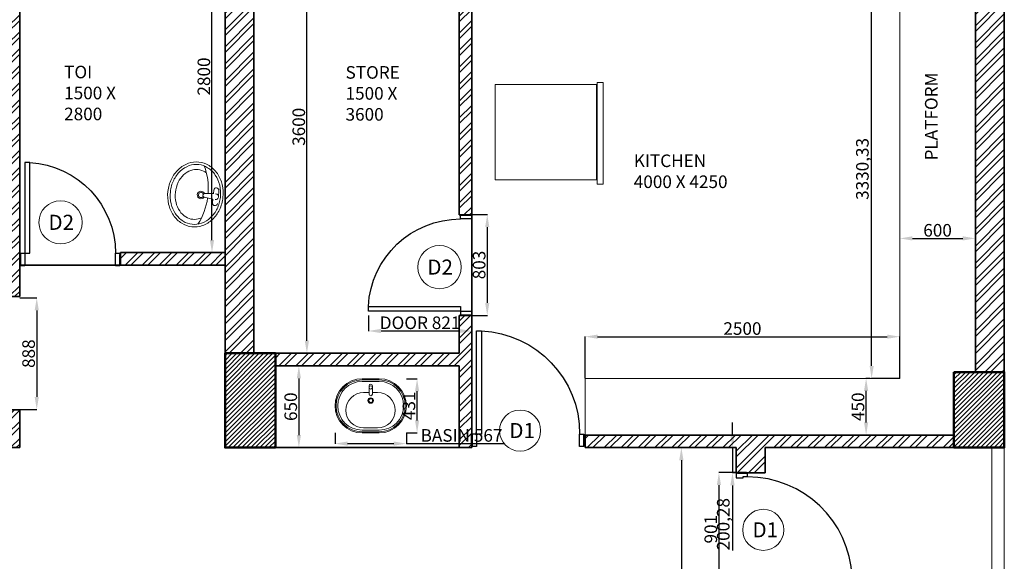
# Model space of a CAD drawing. Units: millimetres. Extents: x -3326 to 29338, y -16792 to 6002.
# Tile 20 of 21: x 21462 to 29282, y -3388 to 918. Entities that reach past the tile are written whole.
import ezdxf

# ---------------------------------------------------------------- set-up
doc = ezdxf.new("R2010")
doc.units = ezdxf.units.MM
doc.header["$PDMODE"] = 35
doc.header["$PDSIZE"] = 5
for name, color, linetype, lineweight in [('A-ANNO-DIMS', 2, 'Continuous', 13), ('A-ANNO-SYMB', 7, 'Continuous', 18), ('A-AREA-IDEN', 7, 'Continuous', 18), ('A-COLS', 1, 'Continuous', 50), ('A-COLS-PATT', 251, 'Continuous', 13), ('A-DOOR', 3, 'Continuous', 25), ('A-EQPM', 9, 'Continuous', 18), ('A-FLOR-CASE', 30, 'Continuous', 18), ('A-FLOR-FIXT', 9, 'Continuous', 18), ('A-FLOR-RAIL', 8, 'Continuous', 20), ('A-WALL', 7, 'Continuous', 35), ('A-WALL-PATT', 252, 'Continuous', 13), ('txt', 7, 'Continuous', 18)]:
    doc.layers.add(name, color=color, linetype=linetype, lineweight=lineweight)
doc.styles.get("Standard").update_dxf_attribs({"font": 'arial.ttf'})
doc.dimstyles.new('ISO-25', dxfattribs={"dimtxt": 100, "dimasz": 100, "dimexe": 1.25, "dimexo": 0.625, "dimtad": 1, "dimtxsty": 'Standard', "dimcen": 2.5, "dimadec": 0, "dimazin": 0, "dimtfac": 1, "dimtmove": 0, "dimatfit": 3, "dimfxl": 1, "dimarcsym": 0})
pattern_1 = [(45, (-10476.65, 1e-12), (-67.35192, 67.35192), []), (45, (-10431.74, 1e-12), (-67.35192, 67.35192), [])]

# ---------------------------------------------------------------- blocks, each defined once
blk = doc.blocks.new('A$C13FC179C')
for points in [[(993.9, 100), (920, 100), (920, 1020), (960, 1020), (960, 100), (960, 60), (947.8, 60), (947.8, 0), (993.9, 0)], [(6.1, 0), (46.1, 0), (46.1, 60), (33.9, 60), (33.9, 100), (6.1, 100)], [(6.1, 100), (6.1, 0)], [(993.9, 100), (993.9, 0)]]:
    blk.add_lwpolyline(points)
for points in [[(0, 10), (6.1, 10), (6.1, 90), (0, 90)], [(993.9, 10), (1000, 10), (1000, 90), (993.9, 90)]]:
    blk.add_lwpolyline(points, close=True)
blk.add_arc((960, 100), 920.9, 92.48955, 180)
blk = doc.blocks.new('A$C0CE462CD')
for p, q in [((860, 100), (860, 0)), ((860, 0), (893.9, 0))]:
    blk.add_line(p, q)
for points in [[(860, 100), (860, 920), (818.4, 920), (818.4, 100)], [(0, 10), (6.1, 10), (6.1, 90), (0, 90)], [(893.9, 10), (900, 10), (900, 90), (893.9, 90)]]:
    blk.add_lwpolyline(points, close=True)
for points in [[(6.1, 0), (40, 0), (40, 100), (6.1, 100)], [(6.1, 100), (6.1, 0)], [(860, 100), (893.9, 100), (893.9, 0)]]:
    blk.add_lwpolyline(points)
blk.add_arc((859.1, 101.9), 819.1, 92.8508, 180.13091)
blk = doc.blocks.new('A$C6ED17C1F')
for points in [[(793.9, 100), (720, 100), (720, 820), (760, 820), (760, 0), (793.9, 0)], [(6.1, 0), (40, 0), (40, 100), (6.1, 100)], [(6.1, 100), (6.1, 0)], [(793.9, 100), (793.9, 0)]]:
    blk.add_lwpolyline(points)
for points in [[(0, 10), (6.1, 10), (6.1, 90), (0, 90)], [(793.9, 10), (800, 10), (800, 90), (793.9, 90)]]:
    blk.add_lwpolyline(points, close=True)
blk.add_arc((761.2, 100), 721.2, 93.27315, 180)
blk = doc.blocks.new('A$C6B943AC5')
for p, q in [((0.207, 0.401), (0.2589, 0.4042)), ((0.2071, 0.362), (0.2386, 0.3621)), ((0.2361, 0.3625), (0.2439, 0.2926)), ((0.2809, 0.3627), (0.2736, 0.2927)), ((0.3111, 0.3624), (0.2796, 0.3623))]:
    blk.add_line(p, q)
for points in [[(0.518, 0.2209, -0.113917), (0.4993, 0.1385, -0.1036), (0.4427, 0.0651, -0.091717), (0.3606, 0.0176, -0.084781), (0.2598, 0, -0.084781), (0.1587, 0.0169, -0.091717), (0.0764, 0.0638, -0.1036), (0.0193, 0.1368, -0.113917), (0, 0.2191, -0.113917), (0.0187, 0.3015, -0.1036), (0.0753, 0.3749, -0.091717), (0.1574, 0.4224, -0.084781), (0.2582, 0.44, -0.084781), (0.3592, 0.4231, -0.091717), (0.4416, 0.3762, -0.1036), (0.4987, 0.3032, -0.113917)], [(0.498, 0.2208, -0.113917), (0.4813, 0.1472, -0.1036), (0.4297, 0.0803, -0.091717), (0.3539, 0.0364, -0.084781), (0.2597, 0.02, -0.084781), (0.1653, 0.0358, -0.091717), (0.0893, 0.0791, -0.1036), (0.0372, 0.1457, -0.113917), (0.02, 0.2192, -0.113917), (0.0367, 0.2928, -0.1036), (0.0883, 0.3597, -0.091717), (0.1641, 0.4036, -0.084781), (0.2583, 0.42, -0.084781), (0.3527, 0.4042, -0.091717), (0.4287, 0.3609, -0.1036), (0.4808, 0.2943, -0.113917)]]:
    blk.add_lwpolyline(points, format="xyb", close=True)
for points in [[(0.458, 0.2207, -0.113917), (0.4453, 0.1646, -0.1036), (0.4037, 0.1107, -0.091717), (0.3405, 0.0741, -0.084781), (0.2595, 0.06, -0.084781), (0.1785, 0.0736, -0.091717), (0.1151, 0.1097, -0.1036), (0.0731, 0.1633, -0.113917), (0.06, 0.2193, -0.113917), (0.0727, 0.2754, -0.020517), (0.0792, 0.2874, -0.091717)], [(0.4384, 0.2886, -0.020517), (0.4449, 0.2767, -0.113917), (0.458, 0.2207, -0.113917)]]:
    blk.add_lwpolyline(points, format="xyb")
for centre, radius, start, end in [((0.207, 0.3815), 0.0195, 90.19698, 270.19698), ((0.259, 0.3817), 0.0225, 354.08148, 186.31248), ((0.311, 0.3819), 0.0195, 270.19698, 90.19698), ((0.2604, -0.2004), 0.5204, 92.15427, 116.77617), ((0.2604, -0.2004), 0.5204, 63.61779, 88.23969), ((0.2588, 0.265), 0.03, 119.152, 61.24195), ((0.2588, 0.265), 0.02, 116.58131, 63.81265), ((0.2587, 0.295), 0.015, 189.39225, 351.00171)]:
    blk.add_arc(centre, radius, start, end)
blk = doc.blocks.new('A$C6AF055E0')
for p, q in [((0.1999, 0.245), (0.1225, 0.245)), ((0.1999, 0.24), (0.1225, 0.24)), ((0.1999, 0.2325), (0.1225, 0.2325)), ((0.129, 0.1825), (0.1537, 0.1825)), ((0.1537, 0.1758), (0.1537, 0.2135)), ((0.1687, 0.2135), (0.1687, 0.1758)), ((0.1687, 0.1825), (0.1919, 0.1825)), ((0.1225, 0.0125), (0.1999, 0.0125)), ((0.1225, 0.005), (0.1999, 0.005)), ((0.1225, 0), (0.1999, 0)), ((0.129, 0.0225), (0.1919, 0.0225))]:
    blk.add_line(p, q)
for centre, radius in [((0.1612, 0.206), 0.0075), ((0.1612, 0.1463), 0.0125), ((0.1612, 0.1463), 0.0085)]:
    blk.add_circle(centre, radius)
for centre, radius, start, end in [((0.1225, 0.1225), 0.1225, 90, 270), ((0.1225, 0.1225), 0.1175, 90, 270), ((0.1225, 0.1225), 0.11, 90, 270), ((0.1999, 0.1225), 0.1225, 270, 90), ((0.1999, 0.1225), 0.1175, 270, 90), ((0.1999, 0.1225), 0.11, 270, 90), ((0.129, 0.1025), 0.08, 90, 270), ((0.1612, 0.2135), 0.0075, 0, 180), ((0.1919, 0.1025), 0.08, 270, 90), ((0.1612, 0.1758), 0.0075, 180, 0)]:
    blk.add_arc(centre, radius, start, end)
blk = doc.blocks.new('*D95')
at = {"layer": 'A-ANNO-DIMS', "color": 0, "lineweight": -2, "transparency": 16777216}
for p, q in [((27123.4, -2383.7), (27123.4, -2283.7)), ((27151.7, -2483.7), (27122.1, -2483.7)), ((27123.4, -2483.7), (27123.4, -2684)), ((27151.7, -2684), (27122.1, -2684)), ((27123.4, -2784), (27123.4, -3302.3))]:
    blk.add_line(p, q, dxfattribs=at)
at = {"layer": 'A-ANNO-DIMS', "color": 0, "transparency": 16777216}
for points in [[(27106.7, -2383.7), (27140.1, -2383.7), (27123.4, -2483.7)], [(27106.7, -2784), (27140.1, -2784), (27123.4, -2684)]]:
    blk.add_solid(points, dxfattribs=at)
at = {"layer": 'Defpoints', "color": 0, "transparency": 16777216}
for p in [(27152.3, -2483.7), (27123.4, -2684), (27152.3, -2684)]:
    blk.add_point(p, dxfattribs=at)
at = {"layer": 'A-ANNO-DIMS', "color": 0, "transparency": 16777216, "insert": (27062.7, -3093.1), "char_height": 100, "attachment_point": 5, "rotation": 90}
blk.add_mtext('200,28', dxfattribs=at)
blk = doc.blocks.new('*D96')
at = {"layer": 'A-ANNO-DIMS', "color": 0, "lineweight": -2, "transparency": 16777216}
for p, q in [((26717.8, -2484), (26718.5, -2484)), ((26717.2, -2584), (26717.2, -6190.8)), ((26717.8, -6290.8), (26718.5, -6290.8))]:
    blk.add_line(p, q, dxfattribs=at)
at = {"layer": 'A-ANNO-DIMS', "color": 0, "transparency": 16777216}
for points in [[(26700.5, -2584), (26733.9, -2584), (26717.2, -2484)], [(26700.5, -6190.8), (26733.9, -6190.8), (26717.2, -6290.8)]]:
    blk.add_solid(points, dxfattribs=at)
at = {"layer": 'Defpoints', "color": 0, "transparency": 16777216}
for p in [(26717.2, -2484), (26717.2, -6290.8), (26717.2, -6290.8)]:
    blk.add_point(p, dxfattribs=at)
at = {"layer": 'A-ANNO-DIMS', "color": 0, "transparency": 16777216, "insert": (26656.5, -4387.4), "char_height": 100, "attachment_point": 5, "rotation": 90}
blk.add_mtext('3806,82', dxfattribs=at)
blk = doc.blocks.new('*D100')
at = {"layer": 'A-ANNO-DIMS', "color": 0, "lineweight": -2, "transparency": 16777216}
for p, q in [((28452.3, -821.7), (28452.3, -822.3)), ((28552.3, -821), (28952.3, -821)), ((29052.3, -820.4), (29052.3, -819.8))]:
    blk.add_line(p, q, dxfattribs=at)
at = {"layer": 'A-ANNO-DIMS', "color": 0, "transparency": 16777216}
for points in [[(28552.3, -804.4), (28552.3, -837.7), (28452.3, -821)], [(28952.3, -804.4), (28952.3, -837.7), (29052.3, -821)]]:
    blk.add_solid(points, dxfattribs=at)
at = {"layer": 'Defpoints', "color": 0, "transparency": 16777216}
for p in [(28452.3, -821), (29052.3, -821), (29052.3, -821)]:
    blk.add_point(p, dxfattribs=at)
at = {"layer": 'A-ANNO-DIMS', "color": 0, "transparency": 16777216, "insert": (28752.3, -769.4), "char_height": 100, "attachment_point": 5}
blk.add_mtext('600', dxfattribs=at)
blk = doc.blocks.new('*D101')
at = {"layer": 'A-ANNO-DIMS', "color": 0, "lineweight": -2, "transparency": 16777216}
for p, q in [((28215.9, -1934), (28183.4, -1934)), ((28184.7, -2284), (28184.7, -2034)), ((28215.9, -2384), (28183.4, -2384))]:
    blk.add_line(p, q, dxfattribs=at)
at = {"layer": 'A-ANNO-DIMS', "color": 0, "transparency": 16777216}
for points in [[(28168, -2034), (28201.3, -2034), (28184.7, -1934)], [(28168, -2284), (28201.3, -2284), (28184.7, -2384)]]:
    blk.add_solid(points, dxfattribs=at)
at = {"layer": 'Defpoints', "color": 0, "transparency": 16777216}
for p in [(28184.7, -1934), (28216.5, -1934), (28216.5, -2384)]:
    blk.add_point(p, dxfattribs=at)
at = {"layer": 'A-ANNO-DIMS', "color": 0, "transparency": 16777216, "insert": (28133, -2159), "char_height": 100, "attachment_point": 5, "rotation": 90}
blk.add_mtext('450', dxfattribs=at)
blk = doc.blocks.new('*D102')
at = {"layer": 'A-ANNO-DIMS', "color": 0, "lineweight": -2, "transparency": 16777216}
for p, q in [((25952.3, -1933.3), (25952.3, -1600.9)), ((26052.3, -1602.2), (28352.3, -1602.2)), ((28452.3, -1933.3), (28452.3, -1600.9))]:
    blk.add_line(p, q, dxfattribs=at)
at = {"layer": 'A-ANNO-DIMS', "color": 0, "transparency": 16777216}
for points in [[(26052.3, -1585.5), (26052.3, -1618.8), (25952.3, -1602.2)], [(28352.3, -1585.5), (28352.3, -1618.8), (28452.3, -1602.2)]]:
    blk.add_solid(points, dxfattribs=at)
at = {"layer": 'Defpoints', "color": 0, "transparency": 16777216}
for p in [(28452.3, -1602.2), (25952.3, -1934), (28452.3, -1934)]:
    blk.add_point(p, dxfattribs=at)
at = {"layer": 'A-ANNO-DIMS', "color": 0, "transparency": 16777216, "insert": (27202.3, -1550.5), "char_height": 100, "attachment_point": 5}
blk.add_mtext('2500', dxfattribs=at)
blk = doc.blocks.new('*D103')
at = {"layer": 'A-ANNO-DIMS', "color": 0, "lineweight": -2, "transparency": 16777216}
for p, q in [((28451.7, 1396.4), (28227.4, 1396.4)), ((28228.6, -1834), (28228.6, 1296.4)), ((28451.7, -1934), (28227.4, -1934))]:
    blk.add_line(p, q, dxfattribs=at)
at = {"layer": 'A-ANNO-DIMS', "color": 0, "transparency": 16777216}
for points in [[(28212, 1296.4), (28245.3, 1296.4), (28228.6, 1396.4)], [(28212, -1834), (28245.3, -1834), (28228.6, -1934)]]:
    blk.add_solid(points, dxfattribs=at)
at = {"layer": 'Defpoints', "color": 0, "transparency": 16777216}
for p in [(28228.6, 1396.4), (28452.3, 1396.4), (28452.3, -1934)]:
    blk.add_point(p, dxfattribs=at)
at = {"layer": 'A-ANNO-DIMS', "color": 0, "transparency": 16777216, "insert": (28167.9, -268.8), "char_height": 100, "attachment_point": 5, "rotation": 90}
blk.add_mtext('3330,33', dxfattribs=at)
blk = doc.blocks.new('*D112')
at = {"layer": 'A-ANNO-DIMS', "color": 0, "lineweight": -2, "transparency": 16777216}
for p, q in [((23743.4, 1866), (23744, 1866)), ((23742.8, -1634), (23742.8, 1766)), ((23743.4, -1734), (23744, -1734))]:
    blk.add_line(p, q, dxfattribs=at)
at = {"layer": 'A-ANNO-DIMS', "color": 0, "transparency": 16777216}
for points in [[(23726.1, 1766), (23759.4, 1766), (23742.8, 1866)], [(23726.1, -1634), (23759.4, -1634), (23742.8, -1734)]]:
    blk.add_solid(points, dxfattribs=at)
at = {"layer": 'Defpoints', "color": 0, "transparency": 16777216}
for p in [(23742.8, 1866), (23742.8, 1866), (23742.8, -1734)]:
    blk.add_point(p, dxfattribs=at)
at = {"layer": 'A-ANNO-DIMS', "color": 0, "transparency": 16777216, "insert": (23691.1, 66), "char_height": 100, "attachment_point": 5, "rotation": 90}
blk.add_mtext('3600', dxfattribs=at)
blk = doc.blocks.new('*D114')
at = {"layer": 'A-ANNO-DIMS', "color": 0, "lineweight": -2, "transparency": 16777216}
for p, q in [((23091.7, 1866), (22987.8, 1866)), ((22989, -834), (22989, 1766)), ((23091.7, -934), (22987.8, -934))]:
    blk.add_line(p, q, dxfattribs=at)
at = {"layer": 'A-ANNO-DIMS', "color": 0, "transparency": 16777216}
for points in [[(22972.4, 1766), (23005.7, 1766), (22989, 1866)], [(22972.4, -834), (23005.7, -834), (22989, -934)]]:
    blk.add_solid(points, dxfattribs=at)
at = {"layer": 'Defpoints', "color": 0, "transparency": 16777216}
for p in [(22989, 1866), (23092.3, 1866), (23092.3, -934)]:
    blk.add_point(p, dxfattribs=at)
at = {"layer": 'A-ANNO-DIMS', "color": 0, "transparency": 16777216, "insert": (22937.4, 466), "char_height": 100, "attachment_point": 5, "rotation": 90}
blk.add_mtext('2800', dxfattribs=at)
blk = doc.blocks.new('*D151')
at = {"layer": 'A-ANNO-DIMS', "color": 0, "lineweight": -2, "transparency": 16777216}
for p, q in [((23492.9, -1834), (23680.3, -1834)), ((23679.1, -1934), (23679.1, -2384)), ((23492.9, -2484), (23680.3, -2484))]:
    blk.add_line(p, q, dxfattribs=at)
at = {"layer": 'A-ANNO-DIMS', "color": 0, "transparency": 16777216}
for points in [[(23662.4, -1934), (23695.8, -1934), (23679.1, -1834)], [(23662.4, -2384), (23695.8, -2384), (23679.1, -2484)]]:
    blk.add_solid(points, dxfattribs=at)
at = {"layer": 'Defpoints', "color": 0, "transparency": 16777216}
for p in [(23492.3, -1834), (23492.3, -2484), (23679.1, -2484)]:
    blk.add_point(p, dxfattribs=at)
at = {"layer": 'A-ANNO-DIMS', "color": 0, "transparency": 16777216, "insert": (23627.4, -2159), "char_height": 100, "attachment_point": 5, "rotation": 90}
blk.add_mtext('650', dxfattribs=at)
blk = doc.blocks.new('REFRIGERATOR-PLAN')
for points in [[(0, 791.3), (804.9, 791.3), (804.9, 34.9), (0, 34.9)], [(812.5, 807.8), (859.3, 807.8), (859.3, 0), (812.5, 0)]]:
    blk.add_lwpolyline(points, close=True)
blk = doc.blocks.new('TAG-D1')
blk.add_circle((163.3, 163.3), 163.3)
at = {"insert": (78, 223.5), "char_height": 120, "attachment_point": 1}
blk.add_mtext_dynamic_manual_height_columns('D1', width=137.943, gutter_width=12.5, heights=[0], dxfattribs=at)
blk = doc.blocks.new('TAG-D2')
blk.add_circle((172, 172), 172)
at = {"insert": (75.7, 232.2), "char_height": 120, "attachment_point": 1}
blk.add_mtext_dynamic_manual_height_columns('D2', width=130.724, gutter_width=12.5, heights=[0], dxfattribs=at)
blk = doc.blocks.new('*D185')
at = {"layer": 'A-ANNO-DIMS', "color": 0, "lineweight": -2, "transparency": 16777216}
for p, q in [((24231.5, -1434.6), (24231.5, -1558.3)), ((25052.3, -1434.6), (25052.3, -1558.3)), ((24952.3, -1557.1), (24331.5, -1557.1))]:
    blk.add_line(p, q, dxfattribs=at)
at = {"layer": 'A-ANNO-DIMS', "color": 0, "transparency": 16777216}
for points in [[(24331.5, -1540.4), (24331.5, -1573.7), (24231.5, -1557.1)], [(24952.3, -1540.4), (24952.3, -1573.7), (25052.3, -1557.1)]]:
    blk.add_solid(points, dxfattribs=at)
at = {"layer": 'Defpoints', "color": 0, "transparency": 16777216}
for p in [(24231.5, -1434), (25052.3, -1434), (24231.5, -1557.1)]:
    blk.add_point(p, dxfattribs=at)
at = {"layer": 'A-ANNO-DIMS', "color": 0, "transparency": 16777216, "insert": (24641.9, -1504.7), "char_height": 100, "attachment_point": 5}
blk.add_mtext('DOOR 821', dxfattribs=at)
blk = doc.blocks.new('*D186')
at = {"layer": 'A-ANNO-DIMS', "color": 0, "lineweight": -2, "transparency": 16777216}
for p, q in [((25052.9, -631), (25176.7, -631)), ((25175.4, -731), (25175.4, -1334)), ((25052.9, -1434), (25176.7, -1434))]:
    blk.add_line(p, q, dxfattribs=at)
at = {"layer": 'A-ANNO-DIMS', "color": 0, "transparency": 16777216}
for points in [[(25158.7, -731), (25192.1, -731), (25175.4, -631)], [(25158.7, -1334), (25192.1, -1334), (25175.4, -1434)]]:
    blk.add_solid(points, dxfattribs=at)
at = {"layer": 'Defpoints', "color": 0, "transparency": 16777216}
for p in [(25052.3, -631), (25052.3, -1434), (25175.4, -1434)]:
    blk.add_point(p, dxfattribs=at)
at = {"layer": 'A-ANNO-DIMS', "color": 0, "transparency": 16777216, "insert": (25123.7, -1032.5), "char_height": 100, "attachment_point": 5, "rotation": 90}
blk.add_mtext('803', dxfattribs=at)
blk = doc.blocks.new('*D188')
at = {"layer": 'A-ANNO-DIMS', "color": 0, "lineweight": -2, "transparency": 16777216}
for p, q in [((21461.4, -1293), (21598.3, -1293)), ((21597, -1393), (21597, -2081.3)), ((21461.4, -2181.3), (21598.3, -2181.3))]:
    blk.add_line(p, q, dxfattribs=at)
at = {"layer": 'A-ANNO-DIMS', "color": 0, "transparency": 16777216}
for points in [[(21580.4, -1393), (21613.7, -1393), (21597, -1293)], [(21580.4, -2081.3), (21613.7, -2081.3), (21597, -2181.3)]]:
    blk.add_solid(points, dxfattribs=at)
at = {"layer": 'Defpoints', "color": 0, "transparency": 16777216}
for p in [(21460.8, -1293), (21460.8, -2181.3), (21597, -2181.3)]:
    blk.add_point(p, dxfattribs=at)
at = {"layer": 'A-ANNO-DIMS', "color": 0, "transparency": 16777216, "insert": (21545.3, -1737.2), "char_height": 100, "attachment_point": 5, "rotation": 90}
blk.add_mtext('888', dxfattribs=at)
blk = doc.blocks.new('*D202')
at = {"layer": 'A-ANNO-DIMS', "color": 0, "lineweight": -2, "transparency": 16777216}
for p, q in [((27152.7, -2681.9), (27014.2, -2681.9)), ((27015.4, -2781.9), (27015.4, -3483.3)), ((27152.7, -3583.3), (27014.2, -3583.3))]:
    blk.add_line(p, q, dxfattribs=at)
at = {"layer": 'A-ANNO-DIMS', "color": 0, "transparency": 16777216}
for points in [[(26998.8, -2781.9), (27032.1, -2781.9), (27015.4, -2681.9)], [(26998.8, -3483.3), (27032.1, -3483.3), (27015.4, -3583.3)]]:
    blk.add_solid(points, dxfattribs=at)
at = {"layer": 'Defpoints', "color": 0, "transparency": 16777216}
for p in [(27153.3, -2681.9), (27015.4, -3583.3), (27153.3, -3583.3)]:
    blk.add_point(p, dxfattribs=at)
at = {"layer": 'A-ANNO-DIMS', "color": 0, "transparency": 16777216, "insert": (26963.7, -3132.6), "char_height": 100, "attachment_point": 5, "rotation": 90}
blk.add_mtext('901', dxfattribs=at)
blk = doc.blocks.new('*D219')
at = {"layer": 'A-ANNO-DIMS', "color": 0, "lineweight": -2, "transparency": 16777216}
for p, q in [((23966.2, -2367.9), (23966.2, -2453.5)), ((24533, -2367.9), (24533, -2453.5)), ((24066.2, -2452.3), (24433, -2452.3)), ((24533, -2452.3), (25308.8, -2452.3))]:
    blk.add_line(p, q, dxfattribs=at)
at = {"layer": 'A-ANNO-DIMS', "color": 0, "transparency": 16777216}
for points in [[(24066.2, -2435.6), (24066.2, -2469), (23966.2, -2452.3)], [(24433, -2435.6), (24433, -2469), (24533, -2452.3)]]:
    blk.add_solid(points, dxfattribs=at)
at = {"layer": 'Defpoints', "color": 0, "transparency": 16777216}
for p in [(23966.2, -2367.3), (24533, -2367.3), (24533, -2452.3)]:
    blk.add_point(p, dxfattribs=at)
at = {"layer": 'A-ANNO-DIMS', "color": 0, "transparency": 16777216, "insert": (24970.9, -2400), "char_height": 100, "attachment_point": 5}
blk.add_mtext('BASIN 567', dxfattribs=at)
blk = doc.blocks.new('*D220')
at = {"layer": 'A-ANNO-DIMS', "color": 0, "lineweight": -2, "transparency": 16777216}
for p, q in [((24533.6, -1936.6), (24619.2, -1936.6)), ((24618, -2267.3), (24618, -2036.6)), ((24533.6, -2367.3), (24619.2, -2367.3))]:
    blk.add_line(p, q, dxfattribs=at)
at = {"layer": 'A-ANNO-DIMS', "color": 0, "transparency": 16777216}
for points in [[(24601.3, -2036.6), (24634.6, -2036.6), (24618, -1936.6)], [(24601.3, -2267.3), (24634.6, -2267.3), (24618, -2367.3)]]:
    blk.add_solid(points, dxfattribs=at)
at = {"layer": 'Defpoints', "color": 0, "transparency": 16777216}
for p in [(24533, -1936.6), (24618, -1936.6), (24533, -2367.3)]:
    blk.add_point(p, dxfattribs=at)
at = {"layer": 'A-ANNO-DIMS', "color": 0, "transparency": 16777216, "insert": (24566.3, -2151.9), "char_height": 100, "attachment_point": 5, "rotation": 90}
blk.add_mtext('431', dxfattribs=at)

msp = doc.modelspace()

# ---------------------------------------------------------------- hatches: boundary and pattern name
at = {"layer": 'A-COLS-PATT'}
h = msp.add_hatch(dxfattribs=at)
h.set_pattern_fill('ANSI31', color=256, scale=8)
h.set_pattern_definition([(45, (-18946.33, 8435.585), (-17.960512, 17.960512), [])])
h.paths.add_polyline_path([(23492.301, -1733.952), (23092.301, -1733.952), (23092.301, -2483.952), (23492.301, -2483.952)])
h = msp.add_hatch(dxfattribs=at)
h.set_pattern_fill('ANSI31', color=256, scale=8)
h.set_pattern_definition([(45, (-12839, 4723.329), (-17.960512, 17.960512), [])])
h.paths.add_polyline_path([(28882.301, -2483.676), (29282.301, -2483.676), (29282.301, -1883.676), (28882.301, -1883.676)])
at = {"layer": 'A-WALL-PATT'}
h = msp.add_hatch(dxfattribs=at)
h.set_pattern_fill('ANSI32', color=256, scale=10)
h.set_pattern_definition(pattern_1)
h.paths.add_polyline_path([(29282.301, -7283.952), (28882.301, -7283.952), (28882.301, -7383.952), (29052.301, -7383.952), (29052.301, -10763.952), (29282.301, -10763.952)])
h.paths.add_polyline_path([(29282.301, -11263.952), (29052.301, -11263.952), (29052.301, -12763.952), (29282.301, -12763.952)])
h.paths.add_polyline_path([(25052.301, -11263.952), (25652.301, -11263.952), (25652.301, -11123.904), (25652.289, -11123.904), (25652.289, -11033.952), (25052.301, -11033.952), (24572.301, -11033.952), (24572.301, -11263.952), (24822.301, -11263.952), (24822.301, -12763.952), (25052.301, -12763.952)])
h.paths.add_polyline_path([(26902.301, -11033.952), (26552.301, -11033.952), (26552.301, -11263.952), (26902.301, -11263.952)])
h.paths.add_polyline_path([(21992.301, -6683.952), (21362.301, -6683.952), (17512.301, -6683.952), (17512.301, -6783.952), (21362.301, -6783.952), (21992.301, -6783.952)])
h.paths.add_polyline_path([(17512.301, -7283.952), (17282.301, -7283.952), (17282.301, -12163.952), (17512.301, -12163.952), (17512.301, -11263.952), (18112.301, -11263.952), (18112.301, -11033.952), (17512.301, -11033.952)])
h.paths.add_polyline_path([(21462.301, -8211.864), (21462.064, -8211.864), (21462.064, -8142.609), (21462.301, -8133.952), (21362.301, -8133.952), (21362.301, -8233.952), (21362.301, -11033.952), (21162.301, -11033.952), (21162.301, -11263.952), (21362.301, -11263.952), (21362.301, -12763.952), (21592.301, -12763.952), (21592.301, -11263.952), (21992.301, -11263.952), (21992.301, -11033.952), (21592.301, -11033.952), (21462.301, -11033.952)])
h.paths.add_polyline_path([(24152.301, -8133.952), (23322.301, -8133.952), (23322.301, -7433.952), (23092.301, -7433.952), (23092.301, -8133.952), (22241.021, -8133.952), (22241.021, -8142.609), (22241.182, -8142.609), (22241.182, -8211.864), (22241.021, -8233.952), (23092.301, -8233.952), (23092.301, -10513.206), (23322.301, -10513.206), (23322.301, -8233.952), (24152.301, -8233.952)])
h.paths.add_polyline_path([(25052.301, -8233.952), (25052.301, -8133.952), (24952.301, -8133.952), (24952.301, -11033.952), (25052.301, -11033.952)])
h.paths.add_polyline_path([(23972.301, -11033.952), (23493.251, -11033.952), (23493.251, -11263.952), (23972.301, -11263.952)])
h.paths.add_polyline_path([(23092.301, -11033.952), (22592.301, -11033.952), (22592.301, -11263.952), (23092.301, -11263.952)])
h.paths.add_polyline_path([(28882.301, -11033.952), (28702.301, -11033.952), (28702.301, -11263.952), (28882.301, -11263.952)])
h.paths.add_polyline_path([(17512.301, -3883.952), (17387.589, -3883.952), (17387.589, -3888.07), (17282.301, -3888.07), (17282.301, -6683.952), (17512.301, -6683.952)])
h.paths.add_polyline_path([(21462.301, -2183.952), (21362.301, -2183.952), (21362.301, -2383.952), (17282.301, -2383.952), (17282.301, -2483.952), (17512.301, -2483.952), (21462.301, -2483.952)])
h.paths.add_polyline_path([(17512.301, -2483.952), (17282.301, -2483.952), (17282.301, -2833.952), (17512.301, -2833.952)])
h.paths.add_polyline_path([(21462.301, 1866.048), (21992.301, 1866.048), (21992.301, 2096.048), (21592.301, 2096.048), (21592.301, 3596.048), (21362.301, 3596.048), (21362.301, 1866.048), (21362.301, -1283.952), (21462.301, -1283.952)])
h.paths.add_polyline_path([(17512.301, 1496.048), (17282.301, 1496.048), (17282.301, -1983.952), (17612.301, -1983.952), (17612.301, -1883.952), (17512.301, -1883.952)])
h.paths.add_polyline_path([(17512.301, 3596.048), (17282.301, 3596.048), (17282.301, 2096.048), (17512.301, 2096.048)])
h.paths.add_polyline_path([(18135.023, 2096.048), (17685.023, 2096.048), (17685.023, 1866.048), (18135.023, 1866.048), (18135.023, 1876.048), (18128.942, 1876.048), (18128.942, 1956.048), (18135.023, 1956.048)])
h.paths.add_polyline_path([(19385.023, 2096.048), (19035.023, 2096.048), (19035.023, 1866.048), (19385.023, 1866.048)])
h.paths.add_polyline_path([(21362.301, 2096.048), (21185.023, 2096.048), (21185.023, 1866.048), (21362.301, 1866.048)])
h.paths.add_polyline_path([(23092.301, 2096.048), (22592.301, 2096.048), (22592.301, 1866.048), (23092.301, 1866.048)])
h.paths.add_polyline_path([(23972.301, 2096.048), (23492.301, 2096.048), (23492.301, 1866.048), (23972.301, 1866.048)])
h.paths.add_polyline_path([(23972.301, 2496.048), (23872.301, 2496.048), (23872.301, 2096.048), (23972.301, 2096.048)])
h.paths.add_polyline_path([(22692.301, 2496.048), (22592.301, 2496.048), (22592.301, 2096.048), (22692.301, 2096.048)])
h.paths.add_polyline_path([(23322.301, 1346.048), (23092.301, 1346.048), (23092.301, -1733.952), (23322.301, -1733.952)])
h.paths.add_polyline_path([(23092.301, -933.952), (22262.301, -933.952), (22262.301, -1033.952), (23092.301, -1033.952)])
h.paths.add_polyline_path([(24952.301, -1433.952), (24952.301, -1733.952), (23492.301, -1733.952), (23492.301, -1833.952), (24952.301, -1833.952), (24952.301, -2483.952), (25052.301, -2483.952), (25052.301, -2466.23), (25049.26, -2466.23), (25049.26, -2386.23), (25049.941, -1433.952)])
h.paths.add_polyline_path([(22692.301, -11263.952), (22592.301, -11263.952), (22592.301, -11663.952), (22692.301, -11663.952)])
h.paths.add_polyline_path([(23972.301, -11263.952), (23872.301, -11263.952), (23872.301, -11663.952), (23972.301, -11663.952)])
h = msp.add_hatch(dxfattribs=at)
h.set_pattern_fill('ANSI32', color=256, scale=10)
h.set_pattern_definition(pattern_1)
h.paths.add_polyline_path([(29282.301, 3596.048), (29052.301, 3596.048), (29052.301, 2095.065), (29282.301, 2095.065)])
h.paths.add_polyline_path([(25052.301, 3596.048), (24822.301, 3596.048), (24822.301, 2096.048), (24572.301, 2096.048), (24572.301, 1866.048), (24952.301, 1866.048), (24952.301, -633.952), (24972.008, -633.952), (24972.008, -631.026), (25043.379, -631.026), (25052.301, -633.952), (25052.301, 1866.048), (25052.301, 1876.048), (25051.713, 1876.048), (25051.713, 1956.048)])
h.paths.add_polyline_path([(29282.301, 1595.065), (29052.301, 1595.065), (29052.301, -1883.676), (29282.301, -1883.676), (29282.301, 336.048)])
h.paths.add_polyline_path([(28882.301, 2096.048), (27902.301, 2096.048), (27902.301, 1866.048), (28882.301, 1866.048)])
h.paths.add_polyline_path([(26402.301, 2096.048), (25952.301, 2096.048), (25952.301, 1866.048), (26402.301, 1866.048)])
h.paths.add_polyline_path([(28882.301, -2383.952), (25952.301, -2383.952), (25952.301, -2483.952), (27152.301, -2483.952), (27152.301, -2683.952), (27382.301, -2683.952), (27382.301, -2483.952), (28882.301, -2483.952)])

# ---------------------------------------------------------------- linework, layer by layer
at = {"layer": 'A-COLS'}
for points in [[(23092.301, -1733.952), (23492.301, -1733.952), (23492.301, -2483.952), (23092.301, -2483.952)], [(28882.301, -1883.676), (29282.301, -1883.676), (29282.301, -2483.676), (28882.301, -2483.676)]]:
    msp.add_lwpolyline(points, close=True, dxfattribs=at)
at = {"layer": 'A-FLOR-CASE'}
for p, q in [((28452.301, -1933.952), (28452.301, 1266.048)), ((25952.301, -2383.952), (25952.301, -1933.952)), ((25952.301, -1933.952), (28452.301, -1933.952))]:
    msp.add_line(p, q, dxfattribs=at)
at = {"layer": 'A-FLOR-RAIL'}
for p, q in [((29182.301, -2483.676), (29182.301, -6683.952)), ((29282.301, -2483.676), (29282.301, -6683.952))]:
    msp.add_line(p, q, dxfattribs=at)
at = {"layer": 'A-WALL'}
for p, q in [((29282.301, 336.048), (29282.301, 3596.048)), ((21462.301, 1866.048), (21462.301, -1283.952)), ((23092.301, 1866.048), (23092.301, -2483.952)), ((24952.301, 1866.048), (24952.301, -633.952)), ((25052.301, 1866.048), (25052.301, -2483.952)), ((29052.301, 1595.065), (29052.301, -1883.676)), ((23322.301, 1346.048), (23322.301, -1733.952)), ((29282.301, 336.048), (29282.301, -2483.676)), ((24953.374, -633.952), (25052.301, -633.952)), ((23092.301, -933.952), (22262.301, -933.952)), ((22262.301, -933.952), (22262.301, -1033.952)), ((23092.301, -1033.952), (21462.301, -1033.952)), ((21462.301, -1283.952), (21362.301, -1283.952)), ((24952.301, -1433.952), (24952.301, -1733.952)), ((24953.374, -1433.952), (25052.301, -1433.952)), ((24952.301, -1733.952), (23492.301, -1733.952)), ((24952.301, -1833.952), (23492.301, -1833.952)), ((24952.301, -1833.952), (24952.301, -2483.952)), ((21462.301, -2183.952), (21362.301, -2183.952)), ((21462.301, -2183.952), (21462.301, -2483.952)), ((28882.301, -2383.952), (25952.301, -2383.952)), ((25952.301, -2383.952), (25952.301, -2483.952)), ((21462.301, -2483.952), (17512.301, -2483.952)), ((25052.301, -2483.952), (23092.301, -2483.952)), ((27152.301, -2483.952), (25952.301, -2483.952)), ((27152.301, -2483.676), (27152.301, -2683.952)), ((27382.301, -2483.676), (27382.301, -2683.952)), ((29052.301, -2483.952), (27382.301, -2483.952)), ((27382.301, -2683.952), (27152.301, -2683.952))]:
    msp.add_line(p, q, dxfattribs=at)

# ---------------------------------------------------------------- block references
at = {"layer": 'A-ANNO-SYMB'}
for name, p in [('TAG-D2', (21614.301, -865.241)), ('TAG-D2', (24623.732, -1221.338)), ('TAG-D1', (25272.673, -2511.765)), ('TAG-D1', (27204.121, -3301.279))]:
    msp.add_blockref(name, p, dxfattribs=at)
at = {"layer": 'A-DOOR', "xscale": -1}
for name, p in [('A$C6ED17C1F', (22262.301, -1037.979)), ('A$C0CE462CD', (25949.26, -2476.23))]:
    msp.add_blockref(name, p, dxfattribs=at)
at = {"layer": 'A-DOOR'}
for name, p, xscale, yscale, zscale, rotation in [('A$C0CE462CD', (25052.301, -631.026), -0.89213991513551, 0.89213991513551, 0.89213991513551, 90), ('A$C13FC179C', (27153.349, -2681.902), 0.9014347414877603, 0.9014347414877603, 0.9014347414877603, 270)]:
    msp.add_blockref(name, p, dxfattribs=dict(at, xscale=xscale, yscale=yscale, zscale=zscale, rotation=rotation))
at = {"layer": 'A-EQPM'}
msp.add_blockref('REFRIGERATOR-PLAN', (25236.921, -389.136), dxfattribs=at)
at = {"layer": 'A-FLOR-FIXT', "xscale": 999.9999999999998, "yscale": 999.9999999999998, "zscale": 999.9999999999998, "rotation": 263.5597085968623}
msp.add_blockref('A$C6B943AC5', (22667.748, -189.435), dxfattribs=at)
at = {"layer": 'A-FLOR-FIXT', "xscale": 1757.943419899877, "yscale": 1757.943419899877, "zscale": 1757.943419899877}
msp.add_blockref('A$C6AF055E0', (23966.247, -2367.278), dxfattribs=at)

# ---------------------------------------------------------------- texts
at = {"layer": 'A-AREA-IDEN', "char_height": 100, "attachment_point": 1}
for s, width, insert in [('TOI\\P1500 X 2800', 594.84046, (21814.566, 551.624)), ('STORE\\P1500 X 3600', 661.29578, (24049.687, 548.548)), ('KITCHEN\\P4000 X 4250', 1168.90663, (26339.13, -153.899))]:
    msp.add_mtext_dynamic_manual_height_columns(s, width=width, gutter_width=12.5, heights=[0], dxfattribs=dict(at, insert=insert))
at = {"layer": 'txt', "insert": (28652.042, -201.259), "char_height": 100, "attachment_point": 1, "rotation": 90}
msp.add_mtext_dynamic_manual_height_columns('PLATFORM', width=441.09946, gutter_width=12.5, heights=[0], dxfattribs=at)

# ---------------------------------------------------------------- dimensions: what is measured, and where the dimension line sits
at = {"layer": 'A-ANNO-DIMS'}
for base, p1, p2, angle, override, picture, middle in [((22989.037, 1866.048), (23092.301, -933.952), (23092.301, 1866.048), 90, {"dimclrd": 0, "dimclre": 0, "dimclrt": 0}, '*D114', (22937.355, 466.048)), ((23742.77, 1866.048), (23742.77, -1733.952), (23742.77, 1866.048), 90, {"dimclrd": 0, "dimclre": 0, "dimclrt": 0}, '*D112', (23691.053, 66.048)), ((28228.622, 1396.382), (28452.301, -1933.952), (28452.301, 1396.382), 90, {"dimclrd": 0, "dimclre": 0, "dimclrt": 0}, '*D103', (28167.901, -268.785)), ((25175.416, -1433.952), (25052.301, -631.026), (25052.301, -1433.952), 270, {"dimdec": 0, "dimlfac": 1, "dimrnd": 0, "dimzin": 0, "dimdsep": 46, "dimlunit": 2}, '*D186', (25123.7, -1032.489)), ((21597.02, -2181.343), (21460.805, -1292.986), (21460.805, -2181.343), 270, {"dimdec": 0, "dimlfac": 1, "dimrnd": 0, "dimzin": 0, "dimdsep": 46, "dimlunit": 2}, '*D188', (21545.337, -1737.165)), ((23679.088, -2483.952), (23492.301, -1833.952), (23492.301, -2483.952), 90, {"dimclrd": 0, "dimclre": 0, "dimclrt": 0}, '*D151', (23627.406, -2158.952)), ((24617.982, -1936.581), (24532.973, -2367.278), (24532.973, -1936.581), 90, {"dimdec": 0, "dimlfac": 1, "dimrnd": 0, "dimzin": 0, "dimdsep": 46, "dimlunit": 2}, '*D220', (24566.266, -2151.93)), ((28184.659, -1933.952), (28216.516, -2383.952), (28216.516, -1933.952), 90, {"dimclrd": 0, "dimclre": 0, "dimclrt": 0}, '*D101', (28132.977, -2158.952)), ((27123.386, -2683.952), (27152.301, -2483.676), (27152.301, -2683.952), 90, {"dimclrd": 0, "dimclre": 0, "dimclrt": 0}, '*D95', (27062.666, -3093.104)), ((26717.207, -6290.772), (26717.207, -2483.952), (26717.207, -6290.772), 90, {"dimclrd": 0, "dimclre": 0, "dimclrt": 0}, '*D96', (26656.486, -4387.362)), ((27015.43, -3583.337), (27153.349, -2681.902), (27153.349, -3583.337), 270, {"dimdec": 0, "dimlfac": 1, "dimrnd": 0, "dimzin": 0, "dimdsep": 46, "dimlunit": 2}, '*D202', (26963.747, -3132.62))]:
    dim = msp.add_linear_dim(base=base, p1=p1, p2=p2, angle=angle, dimstyle='ISO-25', override=override, dxfattribs=at)
    dim.commit()
    dim.dimension.update_dxf_attribs({"geometry": picture, "text_midpoint": middle})
for base, p1, p2, picture, middle in [((29052.301, -821.04), (28452.301, -821.04), (29052.301, -821.04), '*D100', (28752.301, -769.358)), ((28452.301, -1602.154), (25952.301, -1933.952), (28452.301, -1933.952), '*D102', (27202.301, -1550.472))]:
    dim = msp.add_linear_dim(base=base, p1=p1, p2=p2, dimstyle='ISO-25', override={"dimclrd": 0, "dimclre": 0, "dimclrt": 0}, dxfattribs=at)
    dim.commit()
    dim.dimension.update_dxf_attribs({"geometry": picture, "text_midpoint": middle})
dim = msp.add_linear_dim(base=(24231.532, -1557.067), p1=(25052.301, -1433.952), p2=(24231.532, -1433.952), angle=180, text='DOOR <>', dimstyle='ISO-25', override={"dimdec": 0, "dimlfac": 1, "dimrnd": 0, "dimzin": 0, "dimdsep": 46, "dimlunit": 2}, dxfattribs=at)
dim.commit()
dim.dimension.update_dxf_attribs({"geometry": '*D185', "text_midpoint": (24641.916, -1504.703)})
dim = msp.add_linear_dim(base=(24532.973, -2452.287), p1=(23966.246, -2367.278), p2=(24532.973, -2367.278), text='BASIN <>', dimstyle='ISO-25', override={"dimdec": 0, "dimlfac": 1, "dimrnd": 0, "dimzin": 0, "dimdsep": 46, "dimlunit": 2}, dxfattribs=at)
dim.commit()
dim.dimension.update_dxf_attribs({"geometry": '*D219', "text_midpoint": (24970.876, -2399.956)})

doc.saveas('drawing.dxf')
